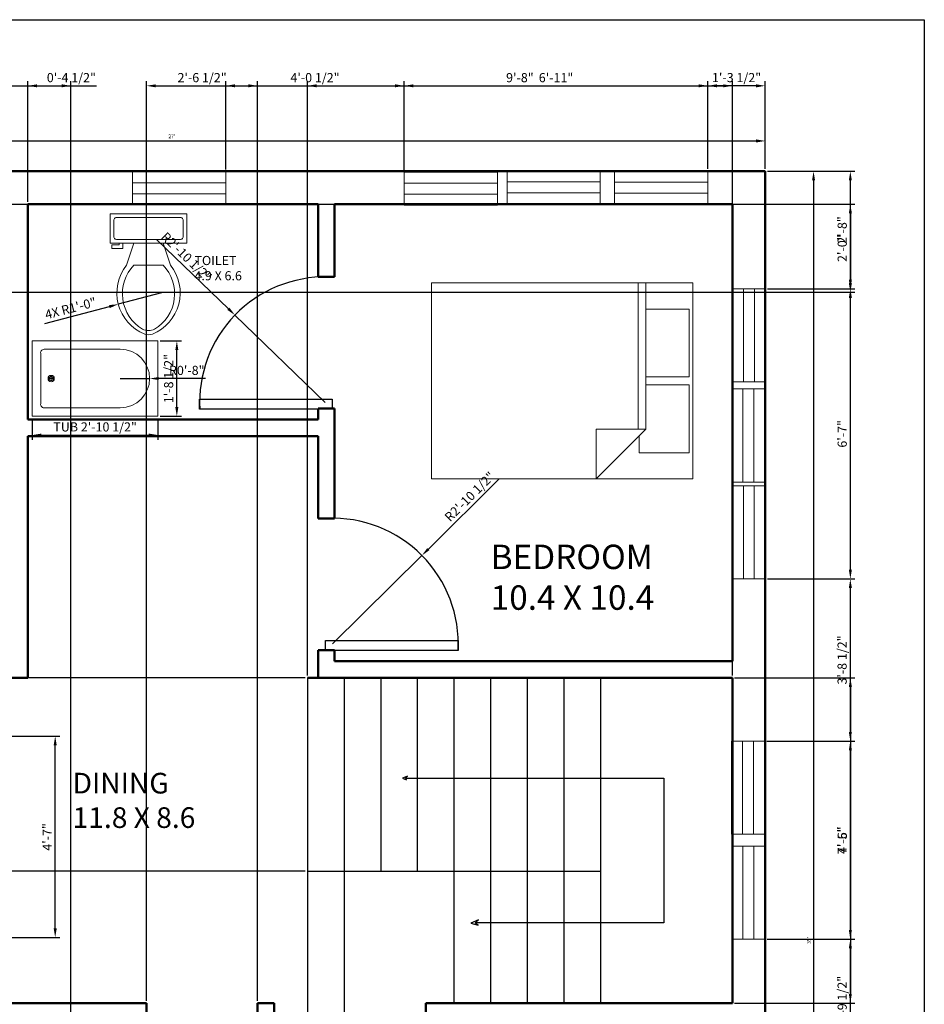
# Model space of a CAD drawing. Units: inches. Extents: x 231 to 633, y -1 to 510.
# Tile 3 of 3: x 386 to 633, y 242 to 510. Entities that reach past the tile are written whole.
import ezdxf

# ---------------------------------------------------------------- set-up
doc = ezdxf.new("R2010")
doc.units = ezdxf.units.IN
for name, color, linetype, lineweight in [('A-ANNO-DIMS', 2, 'Continuous', 18), ('A-ANNO-TTLB', 7, 'Continuous', 25), ('A-AREA-IDEN', 7, 'Continuous', 25), ('A-DOOR', 3, 'Continuous', 25), ('A-FLOR-FIXT', 9, 'Continuous', 18), ('A-FLOR-STRS', 7, 'Continuous', 25), ('A-FURN', 8, 'Continuous', 18), ('A-GLAZ', 4, 'Continuous', 18), ('A-WALL', 7, 'Continuous', 50)]:
    doc.layers.add(name, color=color, linetype=linetype, lineweight=lineweight)
doc.styles.get("Standard").update_dxf_attribs({"font": 'arial.ttf'})
doc.dimstyles.new('ISO-25', dxfattribs={"dimtxt": 2.5, "dimasz": 2.5, "dimexe": 1.25, "dimexo": 0.625, "dimtad": 1, "dimtxsty": 'Standard', "dimcen": 2.5, "dimadec": 0, "dimazin": 0, "dimtfac": 1, "dimtmove": 0, "dimatfit": 3, "dimfxl": 1, "dimarcsym": 0})

# ---------------------------------------------------------------- blocks, each defined once
blk = doc.blocks.new('Toilet - top')
for p, q in [((9.5, -6), (9.5, -2)), ((-8, -8.5), (-8, -8)), ((-7, -8), (-7, -9.5)), ((-4, -8), (-6, -14)), ((4, -8), (6, -14)), ((-10, -8.5), (-8, -8.5)), ((-10, -9.5), (-10, -8.5)), ((-7, -9.5), (-10, -9.5)), ((4, -14), (-4, -14))]:
    blk.add_line(p, q)
blk.add_lwpolyline([(10.5, -8), (10.5, 0), (-10.5, 0), (-10.5, -8)], close=True)
for points in [[(-9.5, -2), (-9.5, -6)], [(8.5, -1), (-8.5, -1)], [(-8.5, -7), (8.5, -7)]]:
    blk.add_lwpolyline(points)
for centre, radius, start, end in [((-8.62, -1.88), 0.884, 81.8699, 188.1301), ((8.62, -1.88), 0.884, 351.8699, 98.1301), ((-8.62, -6.12), 0.884, 171.8699, 278.1301), ((8.62, -6.12), 0.884, 261.8699, 8.1301), ((3.52, -21.58), 12.17, 141.4691, 247.9714), ((4.2, -21.82), 11.33, 136.3677, 238.9468), ((-3.52, -21.58), 12.17, 292.0284, 38.5307), ((-4.2, -21.82), 11.33, 301.053, 43.6321), ((0, -27.88), 4, 245.7318, 294.2682), ((0, -29), 4, 254.8605, 285.1395)]:
    blk.add_arc(centre, radius, start, end)
blk = doc.blocks.new('Bath Tub - 26 x 60 in.')
for p, q in [((8, -18), (10, -18)), ((9, -17), (9, -19))]:
    blk.add_line(p, q)
blk.add_lwpolyline([(0, -36), (0, 0), (60, 0), (60, -36)], close=True)
for points in [[(6, -4), (42, -4)], [(4, -30), (4, -6)], [(42, -32), (6, -32)]]:
    blk.add_lwpolyline(points)
for radius in [1.5, 1]:
    blk.add_circle((9, -18), radius)
for centre, radius, start, end in [((5.75, -5.75), 1.77, 81.8699, 188.1301), ((42, -18), 14, 270, 90), ((5.75, -30.25), 1.77, 171.8699, 278.1301)]:
    blk.add_arc(centre, radius, start, end)
blk = doc.blocks.new('Bed - Queen')
for p, q in [((0, -80.00003), (0, 0)), ((0, 0), (59.99999, 0)), ((59.99999, 0), (59.99999, -80.00003)), ((7.99999, -1.2), (28.79998, -1.2)), ((7.99999, -14.4), (7.99999, -1.2)), ((28.79998, -1.2), (28.79998, -14.4)), ((31.19999, -1.2), (51.99999, -1.2)), ((31.19999, -14.4), (31.19999, -1.2)), ((51.99999, -1.2), (51.99999, -16.4)), ((0, -14.4), (44.8, -14.4)), ((59.99999, -29.6), (44.8, -14.4)), ((44.8, -14.4), (44.8, -29.6)), ((44.8, -16.8), (0, -16.8)), ((51.99999, -16.4), (46.79936, -16.4)), ((44.8, -29.6), (59.99999, -29.6)), ((59.99999, -80.00003), (0, -80.00003))]:
    blk.add_line(p, q)
blk = doc.blocks.new('*D9')
at = {"layer": 'A-ANNO-DIMS', "color": 0, "lineweight": -2, "transparency": 16777216}
for p, q in [((589.91, 469.03), (603.7, 469.03)), ((602.45, 466.53), (602.45, 51.53)), ((589.91, 49.03), (603.7, 49.03))]:
    blk.add_line(p, q, dxfattribs=at)
at = {"layer": 'A-ANNO-DIMS', "color": 0, "transparency": 16777216}
for points in [[(602.04, 466.53), (602.87, 466.53), (602.45, 469.03)], [(602.04, 51.53), (602.87, 51.53), (602.45, 49.03)]]:
    blk.add_solid(points, dxfattribs=at)
at = {"layer": 'Defpoints', "color": 0, "transparency": 16777216}
for p in [(589.28, 469.03), (589.28, 49.03), (602.45, 49.03)]:
    blk.add_point(p, dxfattribs=at)
at = {"layer": 'A-ANNO-DIMS', "color": 0, "transparency": 16777216, "insert": (601.32, 259.03), "char_height": 1, "attachment_point": 5, "rotation": 90}
blk.add_mtext("35'", dxfattribs=at)
blk = doc.blocks.new('*D10')
at = {"layer": 'A-ANNO-DIMS', "color": 0, "lineweight": -2, "transparency": 16777216}
for p, q in [((265.28, 469.66), (265.28, 478.56)), ((589.28, 469.66), (589.28, 478.56)), ((267.78, 477.31), (586.78, 477.31))]:
    blk.add_line(p, q, dxfattribs=at)
at = {"layer": 'A-ANNO-DIMS', "color": 0, "transparency": 16777216}
for points in [[(267.78, 477.73), (267.78, 476.89), (265.28, 477.31)], [(586.78, 477.73), (586.78, 476.89), (589.28, 477.31)]]:
    blk.add_solid(points, dxfattribs=at)
at = {"layer": 'Defpoints', "color": 0, "transparency": 16777216}
for p in [(589.28, 477.31), (265.28, 469.03), (589.28, 469.03)]:
    blk.add_point(p, dxfattribs=at)
at = {"layer": 'A-ANNO-DIMS', "color": 0, "transparency": 16777216, "insert": (427.28, 478.44), "char_height": 1, "attachment_point": 5}
blk.add_mtext("27'", dxfattribs=at)
blk = doc.blocks.new('WIN-25_43x9')
for p, q in [((0, 0), (0, 9)), ((0, 9), (25.43, 9)), ((25.43, 9), (25.43, 0)), ((25.43, 6), (0, 6)), ((0, 3), (25.43, 3)), ((25.43, 0), (0, 0))]:
    blk.add_line(p, q)
blk = doc.blocks.new('*D20')
at = {"layer": 'A-ANNO-DIMS', "color": 0, "lineweight": -2, "transparency": 16777216}
for p, q in [((389.17, 401.52), (389.17, 395.74)), ((423.48, 401.52), (423.48, 395.74)), ((391.67, 396.99), (420.98, 396.99))]:
    blk.add_line(p, q, dxfattribs=at)
at = {"layer": 'A-ANNO-DIMS', "color": 0, "transparency": 16777216}
for points in [[(391.67, 397.41), (391.67, 396.58), (389.17, 396.99)], [(420.98, 397.41), (420.98, 396.58), (423.48, 396.99)]]:
    blk.add_solid(points, dxfattribs=at)
at = {"layer": 'Defpoints', "color": 0, "transparency": 16777216}
for p in [(389.17, 402.14), (423.48, 402.14), (423.48, 396.99)]:
    blk.add_point(p, dxfattribs=at)
at = {"layer": 'A-ANNO-DIMS', "color": 0, "transparency": 16777216, "insert": (406.32, 398.91), "char_height": 2.5, "attachment_point": 5}
blk.add_mtext('TUB 2\'-10 1/2"', dxfattribs=at)
blk = doc.blocks.new('*D21')
at = {"layer": 'A-ANNO-DIMS', "color": 0, "lineweight": -2, "transparency": 16777216}
for p, q in [((424.1, 422.73), (429.88, 422.73)), ((428.63, 404.64), (428.63, 420.23)), ((424.1, 402.14), (429.88, 402.14))]:
    blk.add_line(p, q, dxfattribs=at)
at = {"layer": 'A-ANNO-DIMS', "color": 0, "transparency": 16777216}
for points in [[(428.21, 420.23), (429.04, 420.23), (428.63, 422.73)], [(428.21, 404.64), (429.04, 404.64), (428.63, 402.14)]]:
    blk.add_solid(points, dxfattribs=at)
at = {"layer": 'Defpoints', "color": 0, "transparency": 16777216}
for p in [(423.48, 422.73), (428.63, 422.73), (423.48, 402.14)]:
    blk.add_point(p, dxfattribs=at)
at = {"layer": 'A-ANNO-DIMS', "color": 0, "transparency": 16777216, "insert": (426.71, 412.43), "char_height": 2.5, "attachment_point": 5, "rotation": 90}
blk.add_mtext('1\'-8 1/2"', dxfattribs=at)
blk = doc.blocks.new('*D29')
at = {"layer": 'A-ANNO-DIMS', "color": 0, "lineweight": -2, "transparency": 16777216}
for p, q in [((382.4, 314.78), (396.67, 314.78)), ((395.42, 262.28), (395.42, 312.28)), ((382.4, 259.78), (396.67, 259.78))]:
    blk.add_line(p, q, dxfattribs=at)
at = {"layer": 'A-ANNO-DIMS', "color": 0, "transparency": 16777216}
for points in [[(395.01, 312.28), (395.84, 312.28), (395.42, 314.78)], [(395.01, 262.28), (395.84, 262.28), (395.42, 259.78)]]:
    blk.add_solid(points, dxfattribs=at)
at = {"layer": 'Defpoints', "color": 0, "transparency": 16777216}
for p in [(381.77, 314.78), (395.42, 314.78), (381.77, 259.78)]:
    blk.add_point(p, dxfattribs=at)
at = {"layer": 'A-ANNO-DIMS', "color": 0, "transparency": 16777216, "insert": (393.55, 287.28), "char_height": 2.5, "attachment_point": 5, "rotation": 90}
blk.add_mtext('4\'-7"', dxfattribs=at)
blk = doc.blocks.new('*D33')
at = {"layer": 'A-ANNO-DIMS', "color": 0, "lineweight": -2, "transparency": 16777216}
for p, q in [((464.28, 331.36), (464.28, 493.62)), ((466.78, 492.37), (577.78, 492.37)), ((580.28, 331.36), (580.28, 493.62))]:
    blk.add_line(p, q, dxfattribs=at)
at = {"layer": 'A-ANNO-DIMS', "color": 0, "transparency": 16777216}
for points in [[(466.78, 492.78), (466.78, 491.95), (464.28, 492.37)], [(577.78, 492.78), (577.78, 491.95), (580.28, 492.37)]]:
    blk.add_solid(points, dxfattribs=at)
at = {"layer": 'Defpoints', "color": 0, "transparency": 16777216}
for p in [(580.28, 492.37), (464.28, 330.73), (580.28, 330.73)]:
    blk.add_point(p, dxfattribs=at)
at = {"layer": 'A-ANNO-DIMS', "color": 0, "transparency": 16777216, "insert": (522.28, 494.27), "char_height": 2.5, "attachment_point": 5}
blk.add_mtext('9\'-8"', dxfattribs=at)
blk = doc.blocks.new('*D34')
at = {"layer": 'A-ANNO-DIMS', "color": 0, "lineweight": -2, "transparency": 16777216}
for p, q in [((463.66, 330.73), (240.73, 330.73)), ((241.98, 328.23), (241.98, 280.43)), ((463.66, 277.93), (240.73, 277.93))]:
    blk.add_line(p, q, dxfattribs=at)
at = {"layer": 'A-ANNO-DIMS', "color": 0, "transparency": 16777216}
for points in [[(241.56, 328.23), (242.4, 328.23), (241.98, 330.73)], [(241.56, 280.43), (242.4, 280.43), (241.98, 277.93)]]:
    blk.add_solid(points, dxfattribs=at)
at = {"layer": 'Defpoints', "color": 0, "transparency": 16777216}
for p in [(464.28, 330.73), (241.98, 277.93), (464.28, 277.93)]:
    blk.add_point(p, dxfattribs=at)
at = {"layer": 'A-ANNO-DIMS', "color": 0, "transparency": 16777216, "insert": (240.08, 304.33), "char_height": 2.5, "attachment_point": 5, "rotation": 90}
blk.add_mtext('4\'-5"', dxfattribs=at)
blk = doc.blocks.new('*D35')
at = {"layer": 'A-ANNO-DIMS', "color": 0, "lineweight": -2, "transparency": 16777216}
for p, q in [((464.28, 330.11), (464.28, 4.58)), ((474.28, 330.11), (474.28, 4.58)), ((466.78, 5.83), (471.78, 5.83))]:
    blk.add_line(p, q, dxfattribs=at)
at = {"layer": 'A-ANNO-DIMS', "color": 0, "transparency": 16777216}
for points in [[(466.78, 6.25), (466.78, 5.42), (464.28, 5.83)], [(471.78, 6.25), (471.78, 5.42), (474.28, 5.83)]]:
    blk.add_solid(points, dxfattribs=at)
at = {"layer": 'Defpoints', "color": 0, "transparency": 16777216}
for p in [(464.28, 330.73), (474.28, 330.73), (474.28, 5.83)]:
    blk.add_point(p, dxfattribs=at)
at = {"layer": 'A-ANNO-DIMS', "color": 0, "transparency": 16777216, "insert": (469.28, 7.73), "char_height": 2.5, "attachment_point": 5}
blk.add_mtext('0\'-10"', dxfattribs=at)
blk = doc.blocks.new('*D36')
at = {"layer": 'A-ANNO-DIMS', "color": 0, "lineweight": -2, "transparency": 16777216}
for p, q in [((580.91, 330.73), (613.74, 330.73)), ((612.49, 328.23), (612.49, 244.43)), ((580.91, 241.93), (613.74, 241.93))]:
    blk.add_line(p, q, dxfattribs=at)
at = {"layer": 'A-ANNO-DIMS', "color": 0, "transparency": 16777216}
for points in [[(612.08, 328.23), (612.91, 328.23), (612.49, 330.73)], [(612.08, 244.43), (612.91, 244.43), (612.49, 241.93)]]:
    blk.add_solid(points, dxfattribs=at)
at = {"layer": 'Defpoints', "color": 0, "transparency": 16777216}
for p in [(580.28, 330.73), (580.28, 241.93), (612.49, 241.93)]:
    blk.add_point(p, dxfattribs=at)
at = {"layer": 'A-ANNO-DIMS', "color": 0, "transparency": 16777216, "insert": (610.6, 286.33), "char_height": 2.5, "attachment_point": 5, "rotation": 90}
blk.add_mtext('7\'-5"', dxfattribs=at)
blk = doc.blocks.new('*D38')
at = {"layer": 'A-ANNO-DIMS', "color": 0, "lineweight": -2, "transparency": 16777216}
for p, q in [((380.98, 492.37), (378.48, 492.37)), ((383.48, 460.66), (383.48, 493.62)), ((383.48, 492.37), (387.98, 492.37)), ((387.98, 460.66), (387.98, 493.62)), ((390.48, 492.37), (406.7, 492.37))]:
    blk.add_line(p, q, dxfattribs=at)
at = {"layer": 'A-ANNO-DIMS', "color": 0, "transparency": 16777216}
for points in [[(380.98, 492.78), (380.98, 491.95), (383.48, 492.37)], [(390.48, 492.78), (390.48, 491.95), (387.98, 492.37)]]:
    blk.add_solid(points, dxfattribs=at)
at = {"layer": 'Defpoints', "color": 0, "transparency": 16777216}
for p in [(387.98, 492.37), (383.48, 460.03), (387.98, 460.03)]:
    blk.add_point(p, dxfattribs=at)
at = {"layer": 'A-ANNO-DIMS', "color": 0, "transparency": 16777216, "insert": (399.84, 494.28), "char_height": 2.5, "attachment_point": 5}
blk.add_mtext('0\'-4 1/2"', dxfattribs=at)
blk = doc.blocks.new('*D40')
at = {"layer": 'A-ANNO-DIMS', "color": 0, "lineweight": -2, "transparency": 16777216}
for p, q in [((360.11, 460.03), (613.74, 460.03)), ((612.49, 457.53), (612.49, 438.53)), ((360.11, 436.03), (613.74, 436.03))]:
    blk.add_line(p, q, dxfattribs=at)
at = {"layer": 'A-ANNO-DIMS', "color": 0, "transparency": 16777216}
for points in [[(612.08, 457.53), (612.91, 457.53), (612.49, 460.03)], [(612.08, 438.53), (612.91, 438.53), (612.49, 436.03)]]:
    blk.add_solid(points, dxfattribs=at)
at = {"layer": 'Defpoints', "color": 0, "transparency": 16777216}
for p in [(359.48, 460.03), (359.48, 436.03), (612.49, 436.03)]:
    blk.add_point(p, dxfattribs=at)
at = {"layer": 'A-ANNO-DIMS', "color": 0, "transparency": 16777216, "insert": (610.59, 448.03), "char_height": 2.5, "attachment_point": 5, "rotation": 90}
blk.add_mtext('2\'-0"', dxfattribs=at)
blk = doc.blocks.new('*D53')
at = {"layer": 'A-ANNO-DIMS', "color": 0, "lineweight": -2, "transparency": 16777216}
for p, q in [((589.78, 259.34), (613.74, 259.34)), ((612.49, 228.44), (612.49, 256.84)), ((589.84, 225.94), (613.74, 225.94))]:
    blk.add_line(p, q, dxfattribs=at)
at = {"layer": 'A-ANNO-DIMS', "color": 0, "transparency": 16777216}
for points in [[(612.08, 256.84), (612.91, 256.84), (612.49, 259.34)], [(612.08, 228.44), (612.91, 228.44), (612.49, 225.94)]]:
    blk.add_solid(points, dxfattribs=at)
at = {"layer": 'Defpoints', "color": 0, "transparency": 16777216}
for p in [(589.15, 259.34), (612.49, 259.34), (589.22, 225.94)]:
    blk.add_point(p, dxfattribs=at)
at = {"layer": 'A-ANNO-DIMS', "color": 0, "transparency": 16777216, "insert": (610.58, 242.64), "char_height": 2.5, "attachment_point": 5, "rotation": 90}
blk.add_mtext('2\'-9 1/2"', dxfattribs=at)
blk = doc.blocks.new('*D54')
at = {"layer": 'A-ANNO-DIMS', "color": 0, "lineweight": -2, "transparency": 16777216}
for p, q in [((589.65, 313.45), (613.74, 313.45)), ((612.49, 261.84), (612.49, 310.95)), ((589.78, 259.34), (613.74, 259.34))]:
    blk.add_line(p, q, dxfattribs=at)
at = {"layer": 'A-ANNO-DIMS', "color": 0, "transparency": 16777216}
for points in [[(612.08, 310.95), (612.91, 310.95), (612.49, 313.45)], [(612.08, 261.84), (612.91, 261.84), (612.49, 259.34)]]:
    blk.add_solid(points, dxfattribs=at)
at = {"layer": 'Defpoints', "color": 0, "transparency": 16777216}
for p in [(589.03, 313.45), (612.49, 313.45), (589.15, 259.34)]:
    blk.add_point(p, dxfattribs=at)
at = {"layer": 'A-ANNO-DIMS', "color": 0, "transparency": 16777216, "insert": (610.59, 286.4), "char_height": 2.5, "attachment_point": 5, "rotation": 90}
blk.add_mtext('4\'-6"', dxfattribs=at)
blk = doc.blocks.new('*D55')
at = {"layer": 'A-ANNO-DIMS', "color": 0, "lineweight": -2, "transparency": 16777216}
for p, q in [((589.91, 357.73), (613.74, 357.73)), ((612.49, 315.95), (612.49, 355.23)), ((589.65, 313.45), (613.74, 313.45))]:
    blk.add_line(p, q, dxfattribs=at)
at = {"layer": 'A-ANNO-DIMS', "color": 0, "transparency": 16777216}
for points in [[(612.08, 355.23), (612.91, 355.23), (612.49, 357.73)], [(612.08, 315.95), (612.91, 315.95), (612.49, 313.45)]]:
    blk.add_solid(points, dxfattribs=at)
at = {"layer": 'Defpoints', "color": 0, "transparency": 16777216}
for p in [(589.28, 357.73), (612.49, 357.73), (589.03, 313.45)]:
    blk.add_point(p, dxfattribs=at)
at = {"layer": 'A-ANNO-DIMS', "color": 0, "transparency": 16777216, "insert": (610.57, 335.59), "char_height": 2.5, "attachment_point": 5, "rotation": 90}
blk.add_mtext('3\'-8 1/2"', dxfattribs=at)
blk = doc.blocks.new('*D56')
at = {"layer": 'A-ANNO-DIMS', "color": 0, "lineweight": -2, "transparency": 16777216}
for p, q in [((589.92, 436.95), (613.74, 436.95)), ((612.49, 360.23), (612.49, 434.45)), ((589.91, 357.73), (613.74, 357.73))]:
    blk.add_line(p, q, dxfattribs=at)
at = {"layer": 'A-ANNO-DIMS', "color": 0, "transparency": 16777216}
for points in [[(612.08, 434.45), (612.91, 434.45), (612.49, 436.95)], [(612.08, 360.23), (612.91, 360.23), (612.49, 357.73)]]:
    blk.add_solid(points, dxfattribs=at)
at = {"layer": 'Defpoints', "color": 0, "transparency": 16777216}
for p in [(589.29, 436.95), (612.49, 436.95), (589.28, 357.73)]:
    blk.add_point(p, dxfattribs=at)
at = {"layer": 'A-ANNO-DIMS', "color": 0, "transparency": 16777216, "insert": (610.59, 397.34), "char_height": 2.5, "attachment_point": 5, "rotation": 90}
blk.add_mtext('6\'-7"', dxfattribs=at)
blk = doc.blocks.new('*D57')
at = {"layer": 'A-ANNO-DIMS', "color": 0, "lineweight": -2, "transparency": 16777216}
for p, q in [((589.91, 469.03), (613.74, 469.03)), ((612.49, 439.45), (612.49, 466.53)), ((589.92, 436.95), (613.74, 436.95))]:
    blk.add_line(p, q, dxfattribs=at)
at = {"layer": 'A-ANNO-DIMS', "color": 0, "transparency": 16777216}
for points in [[(612.08, 466.53), (612.91, 466.53), (612.49, 469.03)], [(612.08, 439.45), (612.91, 439.45), (612.49, 436.95)]]:
    blk.add_solid(points, dxfattribs=at)
at = {"layer": 'Defpoints', "color": 0, "transparency": 16777216}
for p in [(589.28, 469.03), (612.49, 469.03), (589.29, 436.95)]:
    blk.add_point(p, dxfattribs=at)
at = {"layer": 'A-ANNO-DIMS', "color": 0, "transparency": 16777216, "insert": (610.59, 452.99), "char_height": 2.5, "attachment_point": 5, "rotation": 90}
blk.add_mtext('2\'-8"', dxfattribs=at)
blk = doc.blocks.new('*D58')
at = {"layer": 'A-ANNO-DIMS', "color": 0, "lineweight": -2, "transparency": 16777216}
for p, q in [((573.57, 469.66), (573.57, 493.62)), ((586.78, 492.37), (576.07, 492.37)), ((589.28, 469.66), (589.28, 493.62))]:
    blk.add_line(p, q, dxfattribs=at)
at = {"layer": 'A-ANNO-DIMS', "color": 0, "transparency": 16777216}
for points in [[(576.07, 492.78), (576.07, 491.95), (573.57, 492.37)], [(586.78, 492.78), (586.78, 491.95), (589.28, 492.37)]]:
    blk.add_solid(points, dxfattribs=at)
at = {"layer": 'Defpoints', "color": 0, "transparency": 16777216}
for p in [(573.57, 492.37), (573.57, 469.04), (589.28, 469.03)]:
    blk.add_point(p, dxfattribs=at)
at = {"layer": 'A-ANNO-DIMS', "color": 0, "transparency": 16777216, "insert": (581.43, 494.29), "char_height": 2.5, "attachment_point": 5}
blk.add_mtext('1\'-3 1/2"', dxfattribs=at)
blk = doc.blocks.new('*D59')
at = {"layer": 'A-ANNO-DIMS', "color": 0, "lineweight": -2, "transparency": 16777216}
for p, q in [((490.72, 469.41), (490.72, 493.62)), ((493.22, 492.37), (571.07, 492.37)), ((573.57, 469.66), (573.57, 493.62))]:
    blk.add_line(p, q, dxfattribs=at)
at = {"layer": 'A-ANNO-DIMS', "color": 0, "transparency": 16777216}
for points in [[(493.22, 492.78), (493.22, 491.95), (490.72, 492.37)], [(571.07, 492.78), (571.07, 491.95), (573.57, 492.37)]]:
    blk.add_solid(points, dxfattribs=at)
at = {"layer": 'Defpoints', "color": 0, "transparency": 16777216}
for p in [(573.57, 492.37), (490.72, 468.79), (573.57, 469.04)]:
    blk.add_point(p, dxfattribs=at)
at = {"layer": 'A-ANNO-DIMS', "color": 0, "transparency": 16777216, "insert": (532.15, 494.27), "char_height": 2.5, "attachment_point": 5}
blk.add_mtext('6\'-11"', dxfattribs=at)
blk = doc.blocks.new('*D60')
at = {"layer": 'A-ANNO-DIMS', "color": 0, "lineweight": -2, "transparency": 16777216}
for p, q in [((441.98, 469.49), (441.98, 493.62)), ((444.48, 492.37), (488.22, 492.37)), ((490.72, 469.41), (490.72, 493.62))]:
    blk.add_line(p, q, dxfattribs=at)
at = {"layer": 'A-ANNO-DIMS', "color": 0, "transparency": 16777216}
for points in [[(444.48, 492.78), (444.48, 491.95), (441.98, 492.37)], [(488.22, 492.78), (488.22, 491.95), (490.72, 492.37)]]:
    blk.add_solid(points, dxfattribs=at)
at = {"layer": 'Defpoints', "color": 0, "transparency": 16777216}
for p in [(490.72, 492.37), (441.98, 468.86), (490.72, 468.79)]:
    blk.add_point(p, dxfattribs=at)
at = {"layer": 'A-ANNO-DIMS', "color": 0, "transparency": 16777216, "insert": (466.35, 494.28), "char_height": 2.5, "attachment_point": 5}
blk.add_mtext('4\'-0 1/2"', dxfattribs=at)
blk = doc.blocks.new('*D64')
at = {"layer": 'A-ANNO-DIMS', "color": 0, "lineweight": -2, "transparency": 16777216}
for p, q in [((420.38, 242.56), (420.38, 493.62)), ((422.88, 492.37), (448.18, 492.37)), ((450.68, 242.56), (450.68, 493.62))]:
    blk.add_line(p, q, dxfattribs=at)
at = {"layer": 'A-ANNO-DIMS', "color": 0, "transparency": 16777216}
for points in [[(422.88, 492.78), (422.88, 491.95), (420.38, 492.37)], [(448.18, 492.78), (448.18, 491.95), (450.68, 492.37)]]:
    blk.add_solid(points, dxfattribs=at)
at = {"layer": 'Defpoints', "color": 0, "transparency": 16777216}
for p in [(450.68, 492.37), (420.38, 241.93), (450.68, 241.93)]:
    blk.add_point(p, dxfattribs=at)
at = {"layer": 'A-ANNO-DIMS', "color": 0, "transparency": 16777216, "insert": (435.53, 494.28), "char_height": 2.5, "attachment_point": 5}
blk.add_mtext('2\'-6 1/2"', dxfattribs=at)
blk = doc.blocks.new('*D65')
at = {"layer": 'A-ANNO-DIMS', "color": 0, "lineweight": -2, "transparency": 16777216}
for p, q in [((332.78, 116.86), (332.78, 493.62)), ((335.28, 492.37), (397.18, 492.37)), ((399.68, 116.86), (399.68, 493.62))]:
    blk.add_line(p, q, dxfattribs=at)
at = {"layer": 'A-ANNO-DIMS', "color": 0, "transparency": 16777216}
for points in [[(335.28, 492.78), (335.28, 491.95), (332.78, 492.37)], [(397.18, 492.78), (397.18, 491.95), (399.68, 492.37)]]:
    blk.add_solid(points, dxfattribs=at)
at = {"layer": 'Defpoints', "color": 0, "transparency": 16777216}
for p in [(399.68, 492.37), (332.78, 116.23), (399.68, 116.23)]:
    blk.add_point(p, dxfattribs=at)
at = {"layer": 'A-ANNO-DIMS', "color": 0, "transparency": 16777216, "insert": (366.23, 494.26), "char_height": 2.5, "attachment_point": 5}
blk.add_mtext('5\'-7"', dxfattribs=at)
blk = doc.blocks.new('*D67')
at = {"layer": 'A-ANNO-DIMS', "color": 0, "lineweight": -2, "transparency": 16777216}
for p, q in [((423.21, 450.35), (442.7, 431.49)), ((469.15, 405.89), (444.49, 429.75))]:
    blk.add_line(p, q, dxfattribs=at)
at = {"layer": 'A-ANNO-DIMS', "color": 0, "transparency": 16777216}
blk.add_solid([(442.99, 431.79), (442.41, 431.19), (444.49, 429.75)], dxfattribs=at)
at = {"layer": 'Defpoints', "color": 0, "transparency": 16777216}
for p in [(444.49, 429.75), (469.15, 405.89)]:
    blk.add_point(p, dxfattribs=at)
at = {"layer": 'A-ANNO-DIMS', "color": 0, "transparency": 16777216, "insert": (431.03, 445.45), "char_height": 2.5, "attachment_point": 5, "rotation": 315.9296}
blk.add_mtext('R2\'-10 1/2"', dxfattribs=at)
blk = doc.blocks.new('*D68')
at = {"layer": 'A-ANNO-DIMS', "color": 0, "lineweight": -2, "transparency": 16777216}
for p, q in [((516.56, 384.95), (497.3, 365.87)), ((471.15, 339.99), (495.52, 364.12))]:
    blk.add_line(p, q, dxfattribs=at)
at = {"layer": 'A-ANNO-DIMS', "color": 0, "transparency": 16777216}
blk.add_solid([(497.01, 366.17), (497.59, 365.58), (495.52, 364.12)], dxfattribs=at)
at = {"layer": 'Defpoints', "color": 0, "transparency": 16777216}
for p in [(495.52, 364.12), (471.15, 339.99)]:
    blk.add_point(p, dxfattribs=at)
at = {"layer": 'A-ANNO-DIMS', "color": 0, "transparency": 16777216, "insert": (508.8, 379.96), "char_height": 2.5, "attachment_point": 5, "rotation": 44.7118}
blk.add_mtext('R2\'-10 1/2"', dxfattribs=at)
blk = doc.blocks.new('*D74')
at = {"layer": 'A-ANNO-DIMS', "color": 0, "lineweight": -2, "transparency": 16777216}
for p, q in [((424.42, 435.82), (412.65, 432.73)), ((392.57, 427.46), (410.23, 432.1))]:
    blk.add_line(p, q, dxfattribs=at)
at = {"layer": 'A-ANNO-DIMS', "color": 0, "transparency": 16777216}
blk.add_solid([(410.13, 432.5), (410.34, 431.69), (412.65, 432.73)], dxfattribs=at)
at = {"layer": 'Defpoints', "color": 0, "transparency": 16777216}
for p in [(424.42, 435.82), (412.65, 432.73)]:
    blk.add_point(p, dxfattribs=at)
at = {"layer": 'A-ANNO-DIMS', "color": 0, "transparency": 16777216, "insert": (399.71, 431.3), "char_height": 2.5, "attachment_point": 5, "rotation": 14.7187}
blk.add_mtext('4X R1\'-0"', dxfattribs=at)
blk = doc.blocks.new('*D76')
at = {"layer": 'A-ANNO-DIMS', "color": 0, "lineweight": -2, "transparency": 16777216}
for p, q in [((413.18, 412.43), (421.19, 412.43)), ((436.48, 412.44), (423.69, 412.43))]:
    blk.add_line(p, q, dxfattribs=at)
at = {"layer": 'A-ANNO-DIMS', "color": 0, "transparency": 16777216}
blk.add_solid([(423.69, 412.85), (423.69, 412.02), (421.19, 412.43)], dxfattribs=at)
at = {"layer": 'Defpoints', "color": 0, "transparency": 16777216}
for p in [(413.18, 412.43), (421.19, 412.43)]:
    blk.add_point(p, dxfattribs=at)
at = {"layer": 'A-ANNO-DIMS', "color": 0, "transparency": 16777216, "insert": (431.34, 414.34), "char_height": 2.5, "attachment_point": 5, "rotation": 0.002}
blk.add_mtext('R0\'-8"', dxfattribs=at)

msp = doc.modelspace()

# ---------------------------------------------------------------- linework, layer by layer
at = {"layer": 'A-ANNO-TTLB'}
msp.add_lwpolyline([(230.86, 510.42), (632.68, 510.42), (632.68, -0.86), (230.86, -0.86)], close=True, dxfattribs=at)
at = {"layer": 'A-DOOR'}
for points in [[(471.06, 406.81), (471.06, 404.06), (434.85, 404.06), (434.85, 406.81)], [(505.42, 340.95), (505.42, 338.2), (469.22, 338.2), (469.22, 340.95)]]:
    msp.add_lwpolyline(points, close=True, dxfattribs=at)
for centre, radius, start, end in [((469.15, 405.89), 34.31, 88.7872, 183.072), ((471.15, 339.99), 34.3, 356.9465, 92.4767)]:
    msp.add_arc(centre, radius, start, end, dxfattribs=at)
at = {"layer": 'A-FLOR-STRS'}
for p, q in [((464.28, 330.73), (464.28, 277.93)), ((474.28, 330.73), (474.28, 277.93)), ((484.28, 330.73), (484.28, 277.93)), ((494.28, 330.73), (494.28, 277.93)), ((504.28, 330.73), (504.28, 241.93)), ((514.28, 330.73), (514.28, 241.93)), ((524.28, 330.73), (524.28, 241.93)), ((534.28, 330.73), (534.28, 241.93)), ((544.28, 330.73), (544.28, 241.93)), ((491.61, 303.87), (490.22, 303.31)), ((491.05, 303.33), (491.61, 303.87)), ((490.22, 303.31), (491.33, 302.88)), ((491.33, 302.88), (491.03, 303.29)), ((491.04, 303.32), (561.54, 303.32)), ((561.54, 303.32), (561.54, 263.8)), ((464.28, 277.93), (544.28, 277.93)), ((510.99, 264.63), (508.88, 263.7)), ((508.88, 263.7), (510.9, 263.14)), ((510.9, 263.14), (510.04, 263.77)), ((510.06, 263.8), (510.99, 264.63)), ((561.54, 263.8), (510.06, 263.8))]:
    msp.add_line(p, q, dxfattribs=at)
at = {"layer": 'A-WALL'}
for p, q in [((265.28, 469.03), (589.28, 469.03)), ((589.28, 469.03), (589.28, 49.03)), ((387.98, 401.23), (387.98, 460.03)), ((387.98, 460.03), (467.18, 460.03)), ((467.18, 440.23), (467.18, 460.03)), ((471.68, 440.23), (471.68, 460.03)), ((471.68, 460.03), (580.28, 460.03)), ((580.28, 460.03), (580.28, 335.23)), ((467.18, 440.23), (471.68, 440.23)), ((467.18, 404.23), (471.68, 404.23)), ((467.18, 401.23), (467.18, 404.23)), ((471.68, 374.23), (471.68, 404.23)), ((387.98, 401.23), (467.18, 401.23)), ((387.98, 330.73), (387.98, 396.73)), ((387.98, 396.73), (467.18, 396.73)), ((467.18, 374.23), (467.18, 396.73)), ((467.18, 374.23), (471.68, 374.23)), ((467.18, 335.23), (467.18, 338.23)), ((467.18, 338.23), (471.68, 338.23)), ((471.68, 335.23), (471.68, 338.23)), ((467.18, 330.73), (467.18, 335.23)), ((471.68, 335.23), (580.28, 335.23)), ((383.48, 330.73), (387.98, 330.73)), ((464.28, 330.73), (580.28, 330.73)), ((580.28, 330.73), (580.28, 241.93)), ((274.28, 241.93), (420.38, 241.93)), ((420.38, 237.43), (420.38, 241.93)), ((450.68, 241.93), (455.18, 241.93)), ((450.68, 116.23), (450.68, 241.93)), ((455.18, 100.93), (455.18, 241.93)), ((496.58, 241.93), (580.28, 241.93)), ((496.58, 241.93), (496.58, 229.63))]:
    msp.add_line(p, q, dxfattribs=at)

# ---------------------------------------------------------------- block references
at = {"layer": 'A-FLOR-FIXT'}
msp.add_blockref('Toilet - top', (420.9, 457.41), dxfattribs=at)
at = {"layer": 'A-FLOR-FIXT', "xscale": 0.5719035000682604, "yscale": 0.5719035000682604, "zscale": 0.5719035000682604}
msp.add_blockref('Bath Tub - 26 x 60 in.', (389.17, 422.73), dxfattribs=at)
at = {"layer": 'A-FURN', "xscale": 0.8923370876530633, "yscale": 0.8923370876530633, "zscale": 0.8923370876530633, "rotation": 270}
msp.add_blockref('Bed - Queen', (569.52, 438.56), dxfattribs=at)
at = {"layer": 'A-GLAZ'}
for p in [(416.55, 459.86), (490.72, 459.79), (518.8, 460.17), (548.14, 460.04)]:
    msp.add_blockref('WIN-25_43x9', p, dxfattribs=at)
for p, rotation in [((580.29, 436.95), 269.9999999999995), ((580.13, 409.59), 270.0000000000005), ((580.28, 383.16), 269.9999999999991), ((580.03, 313.45), 270.0000000000001), ((580.15, 284.78), 269.9999999999996)]:
    msp.add_blockref('WIN-25_43x9', p, dxfattribs=dict(at, rotation=rotation))

# ---------------------------------------------------------------- texts
at = {"layer": 'A-AREA-IDEN', "attachment_point": 1}
for s, width, gutter_width, insert, char_height in [('TOILET\\P4.9 X 6.6', 21.4243, 12.5, (433.44, 445.92), 2.5), ('BEDROOM\\P10.4 X 10.4', 166.3487, 33.34, (514.32, 367.08), 6.6678), ('DINING\\P11.8 X 8.6', 65.8356, 28.21, (400.18, 304.78), 5.642)]:
    msp.add_mtext_dynamic_manual_height_columns(s, width=width, gutter_width=gutter_width, heights=[0], dxfattribs=dict(at, insert=insert, char_height=char_height))

# ---------------------------------------------------------------- dimensions: what is measured, and where the dimension line sits
at = {"layer": 'A-ANNO-DIMS'}
for base, p1, p2, override, picture, middle in [((387.98, 492.37), (383.48, 460.03), (387.98, 460.03), {"dimdec": 1, "dimlfac": 1, "dimrnd": 0, "dimzin": 1, "dimdsep": 46, "dimlunit": 4, "dimfrac": 2}, '*D38', (399.84, 494.28)), ((450.68, 492.37), (420.38, 241.93), (450.68, 241.93), {"dimdec": 1, "dimlfac": 1, "dimrnd": 0, "dimzin": 1, "dimdsep": 46, "dimlunit": 4, "dimfrac": 2}, '*D64', (435.53, 494.28)), ((490.72, 492.37), (441.98, 468.86), (490.72, 468.79), {"dimdec": 1, "dimlfac": 1, "dimrnd": 0, "dimzin": 1, "dimdsep": 46, "dimlunit": 4, "dimfrac": 2}, '*D60', (466.35, 494.28)), ((573.57, 492.37), (589.28, 469.03), (573.57, 469.04), {"dimdec": 1, "dimlfac": 1, "dimrnd": 0, "dimzin": 1, "dimdsep": 46, "dimlunit": 4, "dimfrac": 2}, '*D58', (581.43, 494.29)), ((399.68, 492.37), (332.78, 116.23), (399.68, 116.23), {"dimdec": 1, "dimlfac": 1, "dimrnd": 0, "dimzin": 1, "dimdsep": 46, "dimlunit": 4, "dimfrac": 2}, '*D65', (366.23, 494.26)), ((580.28, 492.37), (464.28, 330.73), (580.28, 330.73), {"dimdec": 1, "dimlfac": 1, "dimrnd": 0, "dimzin": 1, "dimdsep": 46, "dimlunit": 4, "dimfrac": 2}, '*D33', (522.28, 494.27)), ((573.574, 492.3666), (490.7211, 468.7857), (573.574, 469.0396), {"dimdec": 1, "dimlfac": 1, "dimrnd": 0, "dimzin": 1, "dimdsep": 46, "dimlunit": 4, "dimfrac": 2}, '*D59', (532.1476, 494.268)), ((589.28, 477.31), (265.28, 469.03), (589.28, 469.03), {"dimtxt": 1, "dimdec": 0, "dimlunit": 3, "dimclrd": 0, "dimclre": 0, "dimclrt": 0, "dimtdec": 0}, '*D10', (427.28, 478.44)), ((474.28, 5.83), (464.28, 330.73), (474.28, 330.73), {"dimdec": 1, "dimlfac": 1, "dimrnd": 0, "dimzin": 1, "dimdsep": 46, "dimlunit": 4, "dimfrac": 2}, '*D35', (469.28, 7.73))]:
    dim = msp.add_linear_dim(base=base, p1=p1, p2=p2, dimstyle='ISO-25', override=override, dxfattribs=at)
    dim.commit()
    dim.dimension.update_dxf_attribs({"geometry": picture, "text_midpoint": middle})
for base, p1, p2, override, picture, middle in [((602.45, 49.03), (589.28, 469.03), (589.28, 49.03), {"dimtxt": 1, "dimdec": 0, "dimlunit": 3, "dimclrd": 0, "dimclre": 0, "dimclrt": 0, "dimtdec": 0}, '*D9', (601.32, 259.03)), ((612.49, 469.03), (589.29, 436.95), (589.28, 469.03), {"dimdec": 1, "dimlfac": 1, "dimrnd": 0, "dimzin": 1, "dimdsep": 46, "dimlunit": 4, "dimfrac": 2}, '*D57', (610.59, 452.99)), ((612.49, 436.03), (359.48, 460.03), (359.48, 436.03), {"dimdec": 1, "dimlfac": 1, "dimrnd": 0, "dimzin": 1, "dimdsep": 46, "dimlunit": 4, "dimfrac": 2}, '*D40', (610.59, 448.03)), ((612.49, 436.95), (589.28, 357.73), (589.29, 436.95), {"dimdec": 1, "dimlfac": 1, "dimrnd": 0, "dimzin": 1, "dimdsep": 46, "dimlunit": 4, "dimfrac": 2}, '*D56', (610.59, 397.34)), ((428.63, 422.73), (423.48, 402.14), (423.48, 422.73), {"dimdec": 1, "dimlfac": 1, "dimrnd": 0, "dimzin": 1, "dimdsep": 46, "dimlunit": 4, "dimfrac": 2}, '*D21', (426.71, 412.43)), ((612.49, 357.73), (589.03, 313.45), (589.28, 357.73), {"dimdec": 1, "dimlfac": 1, "dimrnd": 0, "dimzin": 1, "dimdsep": 46, "dimlunit": 4, "dimfrac": 2}, '*D55', (610.57, 335.59)), ((241.98, 277.93), (464.28, 330.73), (464.28, 277.93), {"dimdec": 1, "dimlfac": 1, "dimrnd": 0, "dimzin": 1, "dimdsep": 46, "dimlunit": 4, "dimfrac": 2}, '*D34', (240.08, 304.33)), ((612.49, 241.93), (580.28, 330.73), (580.28, 241.93), {"dimdec": 1, "dimlfac": 1, "dimrnd": 0, "dimzin": 1, "dimdsep": 46, "dimlunit": 4, "dimfrac": 2}, '*D36', (610.6, 286.33)), ((395.42, 314.78), (381.77, 259.78), (381.77, 314.78), {"dimdec": 1, "dimlfac": 1, "dimrnd": 0, "dimzin": 1, "dimdsep": 46, "dimlunit": 4, "dimfrac": 2}, '*D29', (393.55, 287.28)), ((612.49, 313.45), (589.15, 259.34), (589.03, 313.45), {"dimdec": 1, "dimlfac": 1, "dimrnd": 0, "dimzin": 1, "dimdsep": 46, "dimlunit": 4, "dimfrac": 2}, '*D54', (610.59, 286.4)), ((612.49, 259.34), (589.22, 225.94), (589.15, 259.34), {"dimdec": 1, "dimlfac": 1, "dimrnd": 0, "dimzin": 1, "dimdsep": 46, "dimlunit": 4, "dimfrac": 2}, '*D53', (610.58, 242.64))]:
    dim = msp.add_linear_dim(base=base, p1=p1, p2=p2, angle=90, dimstyle='ISO-25', override=override, dxfattribs=at)
    dim.commit()
    dim.dimension.update_dxf_attribs({"geometry": picture, "text_midpoint": middle})
for center, mpoint, picture, middle in [((469.15, 405.89), (444.49, 429.75), '*D67', (429.7, 444.07)), ((471.15, 339.99), (495.52, 364.12), '*D68', (510.15, 378.59))]:
    dim = msp.add_radius_dim(center=center, mpoint=mpoint, dimstyle='ISO-25', override={"dimdec": 1, "dimlfac": 1, "dimrnd": 0, "dimzin": 1, "dimdsep": 46, "dimlunit": 4, "dimfrac": 2}, dxfattribs=at)
    dim.commit()
    dim.dimension.update_dxf_attribs({"geometry": picture, "text_midpoint": middle, "dimtype": 164})
dim = msp.add_radius_dim(center=(424.42, 435.82), mpoint=(412.65, 432.73), text='4X <>', dimstyle='ISO-25', override={"dimdec": 1, "dimlfac": 1, "dimrnd": 0, "dimzin": 1, "dimdsep": 46, "dimlunit": 4, "dimfrac": 2}, dxfattribs=at)
dim.commit()
dim.dimension.update_dxf_attribs({"geometry": '*D74', "text_midpoint": (399.71, 431.3)})
dim = msp.add_radius_dim(center=(413.18, 412.43), mpoint=(421.19, 412.43), dimstyle='ISO-25', override={"dimdec": 1, "dimlfac": 1, "dimrnd": 0, "dimzin": 1, "dimdsep": 46, "dimlunit": 4, "dimfrac": 2}, dxfattribs=at)
dim.commit()
dim.dimension.update_dxf_attribs({"geometry": '*D76', "text_midpoint": (431.34, 414.34)})
dim = msp.add_linear_dim(base=(423.48, 396.99), p1=(389.17, 402.14), p2=(423.48, 402.14), text='TUB <>', dimstyle='ISO-25', override={"dimdec": 1, "dimlfac": 1, "dimrnd": 0, "dimzin": 1, "dimdsep": 46, "dimlunit": 4, "dimfrac": 2}, dxfattribs=at)
dim.commit()
dim.dimension.update_dxf_attribs({"geometry": '*D20', "text_midpoint": (406.32, 398.91)})

doc.saveas('drawing.dxf')
